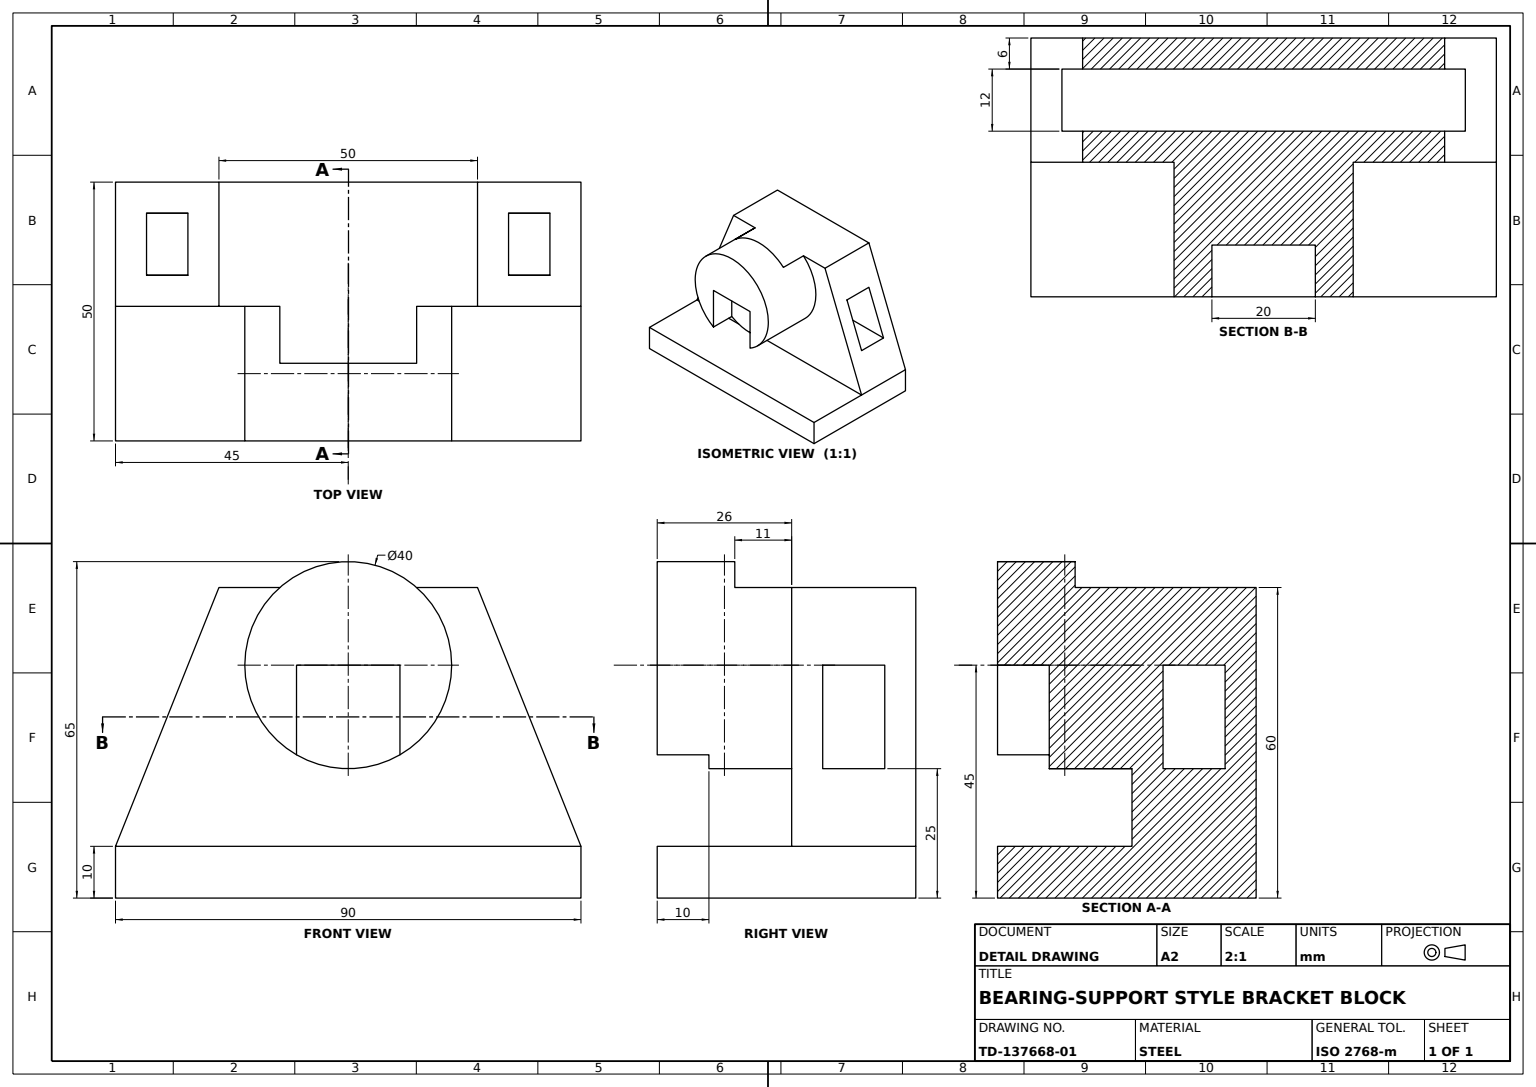
SolidWorks part; units mm, degrees
material "Plain Carbon Steel"
ref_plane "Front Plane" through (0, 0, 0) normal (0, 0, 1) x (1, 0, 0)
ref_plane "Top Plane" through (0, 0, 0) normal (0, 1, 0) x (1, 0, 0)
ref_plane "Right Plane" through (0, 0, 0) normal (1, 0, 0) x (0, 0, -1)
sketch "Support Upright Sketch" plane through (0, 0, 0) normal (0, 0, 1) x (1, 0, 0)
  line L0 (0, 0) -> (0, 10)
  line L1 (0, 10) -> (20, 60)
  line L2 (20, 60) -> (70, 60)
  line L3 (70, 60) -> (90, 10)
  line L4 (90, 10) -> (90, 0)
  line L5 (90, 0) -> (0, 0)
  line L6 (0, 10) -> (90, 10)
  dimension "D1" = 10
  dimension "D2" = 90
  dimension "D3" = 50
  dimension "D4" = 20
  dimension "D5" = 50
extrude "Support Upright" add sketch "Support Upright Sketch" along normal blind 24 contours L1 L6 L3 L2
sketch "Base Plate Sketch" plane through (0, 0, 0) normal (0, 0, 1) x (1, 0, 0)
  line L0 (0, 10) -> (0, 0)
  line L1 (0, 0) -> (90, 0)
  line L2 (90, 0) -> (90, 10)
  line L3 (90, 10) -> (0, 10)
extrude "Base Plate" add sketch "Base Plate Sketch" along normal blind 50
sketch "Bearing Boss Sketch" plane through (0, 0, 24) normal (0, 0, 1) x (1, 0, 0)
  circle A0 centre (45, 45) radius 20
  dimension "D3" = 40
  dimension "D1" = 45
  dimension "D2" = 45
extrude "Bearing Boss Ø40" add sketch "Bearing Boss Sketch" along normal blind 26
sketch "Boss Slot Sketch" plane through (0, 0, 50) normal (0, 0, 1) x (1, 0, 0)
  line L0 (35, 45) -> (55, 45)
  line L1 (55, 45) -> (55, 27.6795)
  line L2 (45, 68.3798) -> (45, 22.6869) construction
  line L3 (35, 45) -> (35, 27.6795)
  circle A0 centre (45, 45) radius 20 construction
  arc A1 (31.7712, 60) -> (58.2288, 60) centre (45, 45) ccw construction
  arc A2 (35, 27.6795) -> (55, 27.6795) centre (45, 45) ccw
  point P10 (45, 45)
  dimension "D1" = 10
extrude "Boss Slot Cut" cut sketch "Boss Slot Sketch" against normal blind 10
sketch "Boss Recess Sketch" plane through (0, 0, 24) normal (0, 0, -1) x (-1, 0, 0)
  line L1 (-58.2288, 60) -> (-31.7712, 60)
  line L2 (-58.2288, 60) -> (-31.7712, 60)
  arc A1 (-31.7712, 60) -> (-58.2288, 60) centre (-45, 45) ccw
  arc A2 (-31.7712, 60) -> (-58.2288, 60) centre (-45, 45) ccw
  dimension "D1" = 0
extrude "Boss Recess Cut" cut sketch "Boss Recess Sketch" against normal blind 11
sketch "Upright Window Sketch" plane through (90, 0, 0) normal (1, 0, 0) x (0, 0, -1)
  line L1 (-18, 45) -> (-6, 45)
  line L2 (-18, 45) -> (-18, 25)
  line L3 (-18, 25) -> (-6, 25)
  line L4 (-6, 45) -> (-6, 25)
  dimension "D1" = 12
  dimension "D2" = 20
  dimension "D3" = 6
  dimension "D4" = 25
extrude "Upright Window 12x20" cut sketch "Upright Window Sketch" against normal through all
